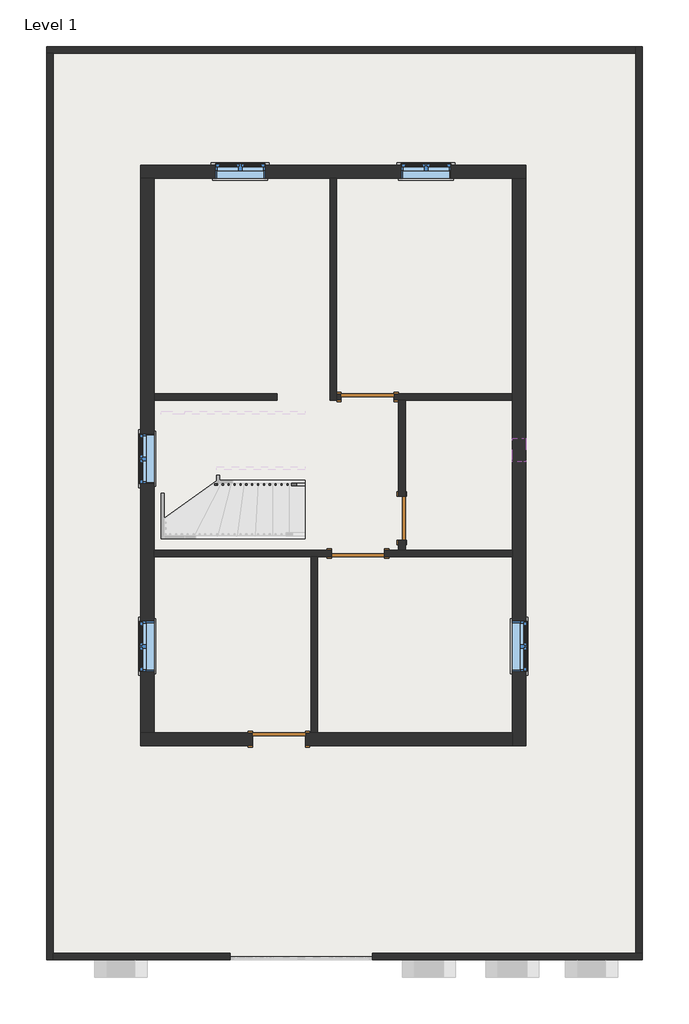
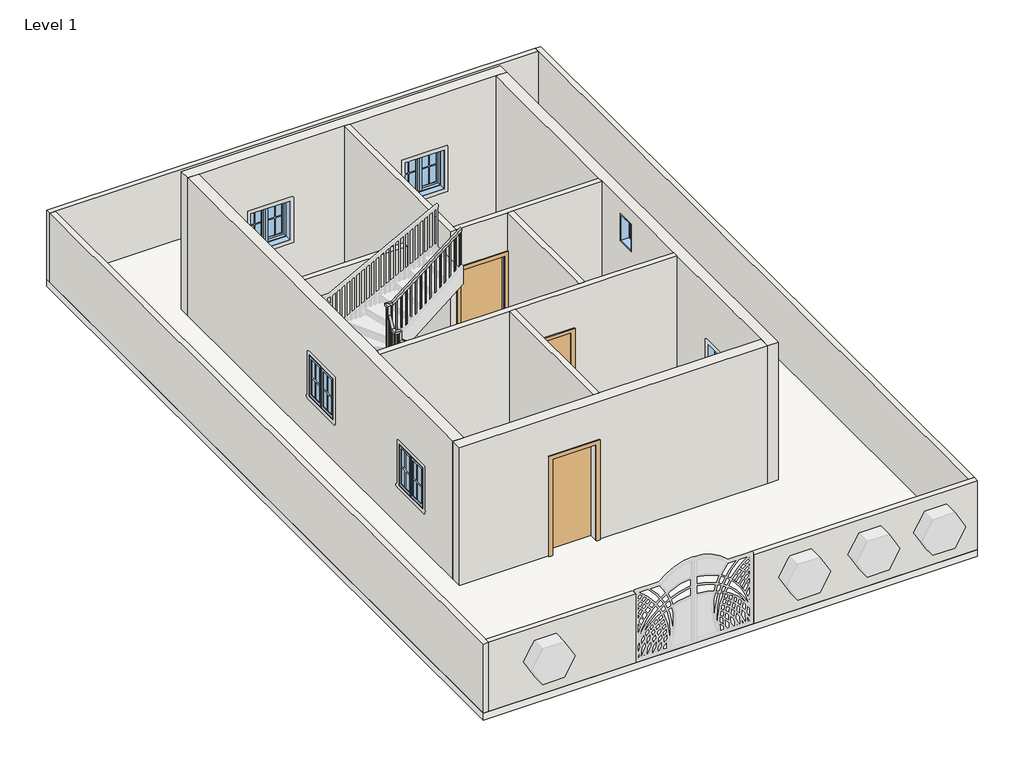
# One storey, part 1 of 2: 15 walls, 6 windows, 4 doors, 1 railing, 1 slab.
"""IFC4 building model written with IfcOpenShell, lengths in millimetres."""

from ifc_helpers import new_model, si_unit, frame, origin, origin_with_axes, place, context, project, spatial, polyline, outline, extrude, faceted_brep, transform, mapped, element, save
from components import door_d8f5dbb5, door_305aa2a5, door_e5f9f3c4, door_a90ba1ad, window_aa618e30, window_339605e1

model = new_model("IFC4")

# Units and contexts
model_context = context("Model", 3, world=origin())
ifc_project = project(units=[si_unit("LENGTHUNIT", "METRE", prefix="MILLI")], contexts=[model_context])

# Site, building, storey
site = spatial("IfcSite", under=ifc_project)
building = spatial("IfcBuilding", under=site)
storey = spatial("IfcBuildingStorey", under=building, Name="Level 1", Elevation=0.0)

# Doors
placement = place(None, origin())
door_shape = door_d8f5dbb5(model_context)
element("IfcDoor", 1, ObjectType="Single-Flush : 30\" x 80\"", at=placement, inside=storey, context=model_context, shape_type="MappedRepresentation", body=[
    mapped(door_shape, transform((-82.2715692, -955.3070853, 0.0), x_axis=(0.0, -1.0, 0.0), y_axis=(1.0, 0.0, 0.0), z_axis=(0.0, 0.0, 1.0))),
])
door_2_shape = door_305aa2a5(model_context)
element("IfcDoor", 2, ObjectType="Single-Flush : 36\" x 84\"", at=placement, inside=storey, context=model_context, shape_type="MappedRepresentation", body=[
    mapped(door_2_shape, transform((-677.5332429, 1140.1929147, 0.0), x_axis=(-1.0, 0.0, 0.0), y_axis=(0.0, -1.0, 0.0), z_axis=(0.0, 0.0, 1.0))),
])
door_3_shape = door_e5f9f3c4(model_context)
element("IfcDoor", 3, ObjectType="Single-Flush : 36\" x 84\"", at=placement, inside=storey, context=model_context, shape_type="MappedRepresentation", body=[
    mapped(door_3_shape, transform((-842.6332429, -1564.9070853, 0.0), x_axis=(-1.0, 0.0, 0.0), y_axis=(0.0, -1.0, 0.0), z_axis=(0.0, 0.0, 1.0))),
])
door_4_shape = door_a90ba1ad(model_context)
element("IfcDoor", 4, ObjectType="Single-Flush : 36\" x 84\"", at=placement, inside=storey, context=model_context, shape_type="MappedRepresentation", body=[
    mapped(door_4_shape, transform((-2212.5949167, -4784.3570853, 0.0), x_axis=(-1.0, 0.0, 0.0), y_axis=(0.0, -1.0, 0.0), z_axis=(0.0, 0.0, 1.0))),
])

# Railing
element("IfcRailing", 5, ObjectType="Handrail - Rectangular", at=placement, inside=storey, context=model_context, shape_type="SolidModel", body=[
    faceted_brep([(-1761.7449167, -396.5070853, 1083.7333333), (-1761.7449167, -396.5070853, 1019.4000346), (-1761.7449167, -345.7070853, 1019.4000346), (-1761.7449167, -345.7070853, 1083.7333333), (-3213.2766085, -396.5070853, 2211.6191036), (-3264.0766085, -396.5070853, 2186.7590024), (-3264.0766085, -345.7070853, 2186.7590024), (-3213.2766085, -345.7070853, 2211.6191036), (-3213.2766085, -396.5070853, 2414.6281882), (-3264.0766085, -396.5070853, 2363.8281882), (-3264.0766085, -345.7070853, 2363.8281882), (-3213.2766085, -345.7070853, 2414.6281882), (-3340.2766085, -396.5070853, 2414.6281882), (-3340.2766085, -396.5070853, 2363.8281882), (-3289.4766085, -345.7070853, 2363.8281882), (-3289.4766085, -345.7070853, 2414.6281882), (-3340.2766085, -269.5070853, 2414.6281882), (-3340.2766085, -240.3857515, 2363.8281882), (-3289.4766085, -240.3857515, 2363.8281882), (-3289.4766085, -269.5070853, 2414.6281882), (-3340.2766085, -142.5070853, 2631.5051451), (-3340.2766085, -91.7070853, 2617.7256424), (-3289.4766085, -91.7070853, 2617.7256424), (-3289.4766085, -142.5070853, 2631.5051451), (-3340.2766085, -142.5070853, 2834.5142297), (-3340.2766085, -91.7070853, 2783.7142297), (-3289.4766085, -91.7070853, 2783.7142297), (-3289.4766085, -142.5070853, 2834.5142297), (-3340.2766085, -15.5070853, 2834.5142297), (-3340.2766085, -15.5070853, 2783.7142297), (-3289.4766085, -66.3070853, 2783.7142297), (-3289.4766085, -66.3070853, 2834.5142297), (-3213.2766085, -15.5070853, 2834.5142297), (-3195.8599406, -15.5070853, 2783.7142297), (-3195.8599406, -66.3070853, 2783.7142297), (-3213.2766085, -66.3070853, 2834.5142297), (-1761.7449167, -15.5070853, 3962.4), (-1761.7449167, -66.3070853, 3962.4), (-1761.7449167, -66.3070853, 3898.0667013), (-1761.7449167, -15.5070853, 3898.0667013)], [[[0, 1, 2, 3]], [[1, 0, 4, 5]], [[2, 1, 5, 6]], [[3, 2, 6, 7]], [[0, 3, 7, 4]], [[5, 4, 8, 9]], [[6, 5, 9, 10]], [[7, 6, 10, 11]], [[4, 7, 11, 8]], [[9, 8, 12, 13]], [[10, 9, 13, 14]], [[11, 10, 14, 15]], [[8, 11, 15, 12]], [[13, 12, 16, 17]], [[14, 13, 17, 18]], [[15, 14, 18, 19]], [[12, 15, 19, 16]], [[17, 16, 20, 21]], [[18, 17, 21, 22]], [[19, 18, 22, 23]], [[16, 19, 23, 20]], [[21, 20, 24, 25]], [[22, 21, 25, 26]], [[23, 22, 26, 27]], [[20, 23, 27, 24]], [[25, 24, 28, 29]], [[26, 25, 29, 30]], [[27, 26, 30, 31]], [[24, 27, 31, 28]], [[29, 28, 32, 33]], [[30, 29, 33, 34]], [[31, 30, 34, 35]], [[28, 31, 35, 32]], [[36, 37, 38, 39]], [[33, 32, 36, 39]], [[34, 33, 39, 38]], [[35, 34, 38, 37]], [[32, 35, 37, 36]]]),
    extrude(outline(polyline([(3882.8316852, -1781.3516085), (3868.0292361, -1800.4016085), (2878.6666667, -1800.4016085), (2878.6666667, -1781.3516085), (3882.8316852, -1781.3516085)])), frame((0.0, -50.4320853, 0.0), z_axis=(0.0, 1.0, 0.0), x_axis=(0.0, 0.0, 1.0)), (0.0, 0.0, 1.0), 19.05),
    extrude(outline(polyline([(3803.8852902, -1882.9516085), (3789.0828411, -1902.0016085), (2878.6666667, -1902.0016085), (2878.6666667, -1882.9516085), (3803.8852902, -1882.9516085)])), frame((0.0, -50.4320853, 0.0), z_axis=(0.0, 1.0, 0.0), x_axis=(0.0, 0.0, 1.0)), (0.0, 0.0, 1.0), 19.05),
    extrude(outline(polyline([(3724.9388952, -1984.5516085), (3710.1364462, -2003.6016085), (2878.6666667, -2003.6016085), (2878.6666667, -1984.5516085), (3724.9388952, -1984.5516085)])), frame((0.0, -50.4320853, 0.0), z_axis=(0.0, 1.0, 0.0), x_axis=(0.0, 0.0, 1.0)), (0.0, 0.0, 1.0), 19.05),
    extrude(outline(polyline([(3645.9925003, -2086.1516085), (3631.1900512, -2105.2016085), (2709.3333333, -2105.2016085), (2709.3333333, -2086.1516085), (3645.9925003, -2086.1516085)])), frame((0.0, -50.4320853, 0.0), z_axis=(0.0, 1.0, 0.0), x_axis=(0.0, 0.0, 1.0)), (0.0, 0.0, 1.0), 19.05),
    extrude(outline(polyline([(3567.0461053, -2187.7516085), (3552.2436562, -2206.8016085), (2709.3333333, -2206.8016085), (2709.3333333, -2187.7516085), (3567.0461053, -2187.7516085)])), frame((0.0, -50.4320853, 0.0), z_axis=(0.0, 1.0, 0.0), x_axis=(0.0, 0.0, 1.0)), (0.0, 0.0, 1.0), 19.05),
    extrude(outline(polyline([(3488.0997103, -2289.3516085), (3473.2972613, -2308.4016085), (2709.3333333, -2308.4016085), (2709.3333333, -2289.3516085), (3488.0997103, -2289.3516085)])), frame((0.0, -50.4320853, 0.0), z_axis=(0.0, 1.0, 0.0), x_axis=(0.0, 0.0, 1.0)), (0.0, 0.0, 1.0), 19.05),
    extrude(outline(polyline([(3409.1533154, -2390.9516085), (3394.3508663, -2410.0016085), (2540.0, -2410.0016085), (2540.0, -2390.9516085), (3409.1533154, -2390.9516085)])), frame((0.0, -50.4320853, 0.0), z_axis=(0.0, 1.0, 0.0), x_axis=(0.0, 0.0, 1.0)), (0.0, 0.0, 1.0), 19.05),
    extrude(outline(polyline([(3330.2069204, -2492.5516085), (3315.4044713, -2511.6016085), (2540.0, -2511.6016085), (2540.0, -2492.5516085), (3330.2069204, -2492.5516085)])), frame((0.0, -50.4320853, 0.0), z_axis=(0.0, 1.0, 0.0), x_axis=(0.0, 0.0, 1.0)), (0.0, 0.0, 1.0), 19.05),
    extrude(outline(polyline([(3251.2605254, -2594.1516085), (3236.4580764, -2613.2016085), (2370.6666667, -2613.2016085), (2370.6666667, -2594.1516085), (3251.2605254, -2594.1516085)])), frame((0.0, -50.4320853, 0.0), z_axis=(0.0, 1.0, 0.0), x_axis=(0.0, 0.0, 1.0)), (0.0, 0.0, 1.0), 19.05),
    extrude(outline(polyline([(3172.3141304, -2695.7516085), (3157.5116814, -2714.8016085), (2370.6666667, -2714.8016085), (2370.6666667, -2695.7516085), (3172.3141304, -2695.7516085)])), frame((0.0, -50.4320853, 0.0), z_axis=(0.0, 1.0, 0.0), x_axis=(0.0, 0.0, 1.0)), (0.0, 0.0, 1.0), 19.05),
    extrude(outline(polyline([(3093.3677355, -2797.3516085), (3078.5652864, -2816.4016085), (2370.6666667, -2816.4016085), (2370.6666667, -2797.3516085), (3093.3677355, -2797.3516085)])), frame((0.0, -50.4320853, 0.0), z_axis=(0.0, 1.0, 0.0), x_axis=(0.0, 0.0, 1.0)), (0.0, 0.0, 1.0), 19.05),
    extrude(outline(polyline([(3014.4213405, -2898.9516085), (2999.6188914, -2918.0016085), (2201.3333333, -2918.0016085), (2201.3333333, -2898.9516085), (3014.4213405, -2898.9516085)])), frame((0.0, -50.4320853, 0.0), z_axis=(0.0, 1.0, 0.0), x_axis=(0.0, 0.0, 1.0)), (0.0, 0.0, 1.0), 19.05),
    extrude(outline(polyline([(2935.4749455, -3000.5516085), (2920.6724965, -3019.6016085), (2201.3333333, -3019.6016085), (2201.3333333, -3000.5516085), (2935.4749455, -3000.5516085)])), frame((0.0, -50.4320853, 0.0), z_axis=(0.0, 1.0, 0.0), x_axis=(0.0, 0.0, 1.0)), (0.0, 0.0, 1.0), 19.05),
    extrude(outline(polyline([(2856.5285506, -3102.1516085), (2841.7261015, -3121.2016085), (2032.0, -3121.2016085), (2032.0, -3102.1516085), (2856.5285506, -3102.1516085)])), frame((0.0, -50.4320853, 0.0), z_axis=(0.0, 1.0, 0.0), x_axis=(0.0, 0.0, 1.0)), (0.0, 0.0, 1.0), 19.05),
    extrude(outline(polyline([(2777.5821556, -3203.7516085), (2762.7797065, -3222.8016085), (2032.0, -3222.8016085), (2032.0, -3203.7516085), (2777.5821556, -3203.7516085)])), frame((0.0, -50.4320853, 0.0), z_axis=(0.0, 1.0, 0.0), x_axis=(0.0, 0.0, 1.0)), (0.0, 0.0, 1.0), 19.05),
    extrude(outline(polyline([(-3305.3516085, -75.8320853), (-3324.4016085, -75.8320853), (-3324.4016085, -56.7820853), (-3305.3516085, -56.7820853), (-3305.3516085, -75.8320853)])), frame((0.0, 0.0, 1693.3333333), z_axis=(0.0, 0.0, 1.0), x_axis=(1.0, 0.0, 0.0)), (0.0, 0.0, 1.0), 1090.3808964),
    extrude(outline(polyline([(-177.4320853, 2471.3336964), (-158.3820853, 2503.86524), (-158.3820853, 1524.0), (-177.4320853, 1524.0), (-177.4320853, 2471.3336964)])), frame((-3324.4016085, 0.0, 0.0), z_axis=(1.0, 0.0, 0.0), x_axis=(0.0, 1.0, 0.0)), (0.0, 0.0, 1.0), 19.05),
    extrude(outline(polyline([(-279.0320853, 2297.8321309), (-259.9820853, 2330.3636744), (-259.9820853, 1354.6666667), (-279.0320853, 1354.6666667), (-279.0320853, 2297.8321309)])), frame((-3324.4016085, 0.0, 0.0), z_axis=(1.0, 0.0, 0.0), x_axis=(0.0, 1.0, 0.0)), (0.0, 0.0, 1.0), 19.05),
    extrude(outline(polyline([(-3276.2199167, -361.5820853), (-3276.2199167, -380.6320853), (-3295.2699167, -380.6320853), (-3295.2699167, -361.5820853), (-3276.2199167, -361.5820853)])), frame((0.0, 0.0, 1185.3333333), z_axis=(0.0, 0.0, 1.0), x_axis=(1.0, 0.0, 0.0)), (0.0, 0.0, 1.0), 1178.4948549),
    extrude(outline(polyline([(2117.2483397, -3174.6199167), (2132.0507888, -3193.6699167), (1016.0, -3193.6699167), (1016.0, -3174.6199167), (2117.2483397, -3174.6199167)])), frame((0.0, -380.6320853, 0.0), z_axis=(0.0, 1.0, 0.0), x_axis=(0.0, 0.0, 1.0)), (0.0, 0.0, 1.0), 19.05),
    extrude(outline(polyline([(2038.3019447, -3073.0199167), (2053.1043938, -3092.0699167), (1016.0, -3092.0699167), (1016.0, -3073.0199167), (2038.3019447, -3073.0199167)])), frame((0.0, -380.6320853, 0.0), z_axis=(0.0, 1.0, 0.0), x_axis=(0.0, 0.0, 1.0)), (0.0, 0.0, 1.0), 19.05),
    extrude(outline(polyline([(1959.3555498, -2971.4199167), (1974.1579988, -2990.4699167), (846.6666667, -2990.4699167), (846.6666667, -2971.4199167), (1959.3555498, -2971.4199167)])), frame((0.0, -380.6320853, 0.0), z_axis=(0.0, 1.0, 0.0), x_axis=(0.0, 0.0, 1.0)), (0.0, 0.0, 1.0), 19.05),
    extrude(outline(polyline([(1880.4091548, -2869.8199167), (1895.2116039, -2888.8699167), (846.6666667, -2888.8699167), (846.6666667, -2869.8199167), (1880.4091548, -2869.8199167)])), frame((0.0, -380.6320853, 0.0), z_axis=(0.0, 1.0, 0.0), x_axis=(0.0, 0.0, 1.0)), (0.0, 0.0, 1.0), 19.05),
    extrude(outline(polyline([(1801.4627598, -2768.2199167), (1816.2652089, -2787.2699167), (677.3333333, -2787.2699167), (677.3333333, -2768.2199167), (1801.4627598, -2768.2199167)])), frame((0.0, -380.6320853, 0.0), z_axis=(0.0, 1.0, 0.0), x_axis=(0.0, 0.0, 1.0)), (0.0, 0.0, 1.0), 19.05),
    extrude(outline(polyline([(1722.5163649, -2666.6199167), (1737.3188139, -2685.6699167), (677.3333333, -2685.6699167), (677.3333333, -2666.6199167), (1722.5163649, -2666.6199167)])), frame((0.0, -380.6320853, 0.0), z_axis=(0.0, 1.0, 0.0), x_axis=(0.0, 0.0, 1.0)), (0.0, 0.0, 1.0), 19.05),
    extrude(outline(polyline([(1643.5699699, -2565.0199167), (1658.3724189, -2584.0699167), (508.0, -2584.0699167), (508.0, -2565.0199167), (1643.5699699, -2565.0199167)])), frame((0.0, -380.6320853, 0.0), z_axis=(0.0, 1.0, 0.0), x_axis=(0.0, 0.0, 1.0)), (0.0, 0.0, 1.0), 19.05),
    extrude(outline(polyline([(1564.6235749, -2463.4199167), (1579.426024, -2482.4699167), (508.0, -2482.4699167), (508.0, -2463.4199167), (1564.6235749, -2463.4199167)])), frame((0.0, -380.6320853, 0.0), z_axis=(0.0, 1.0, 0.0), x_axis=(0.0, 0.0, 1.0)), (0.0, 0.0, 1.0), 19.05),
    extrude(outline(polyline([(1485.6771799, -2361.8199167), (1500.479629, -2380.8699167), (508.0, -2380.8699167), (508.0, -2361.8199167), (1485.6771799, -2361.8199167)])), frame((0.0, -380.6320853, 0.0), z_axis=(0.0, 1.0, 0.0), x_axis=(0.0, 0.0, 1.0)), (0.0, 0.0, 1.0), 19.05),
    extrude(outline(polyline([(1406.730785, -2260.2199167), (1421.533234, -2279.2699167), (338.6666667, -2279.2699167), (338.6666667, -2260.2199167), (1406.730785, -2260.2199167)])), frame((0.0, -380.6320853, 0.0), z_axis=(0.0, 1.0, 0.0), x_axis=(0.0, 0.0, 1.0)), (0.0, 0.0, 1.0), 19.05),
    extrude(outline(polyline([(1327.78439, -2158.6199167), (1342.5868391, -2177.6699167), (338.6666667, -2177.6699167), (338.6666667, -2158.6199167), (1327.78439, -2158.6199167)])), frame((0.0, -380.6320853, 0.0), z_axis=(0.0, 1.0, 0.0), x_axis=(0.0, 0.0, 1.0)), (0.0, 0.0, 1.0), 19.05),
    extrude(outline(polyline([(1248.837995, -2057.0199167), (1263.6404441, -2076.0699167), (338.6666667, -2076.0699167), (338.6666667, -2057.0199167), (1248.837995, -2057.0199167)])), frame((0.0, -380.6320853, 0.0), z_axis=(0.0, 1.0, 0.0), x_axis=(0.0, 0.0, 1.0)), (0.0, 0.0, 1.0), 19.05),
    extrude(outline(polyline([(1169.8916001, -1955.4199167), (1184.6940491, -1974.4699167), (169.3333333, -1974.4699167), (169.3333333, -1955.4199167), (1169.8916001, -1955.4199167)])), frame((0.0, -380.6320853, 0.0), z_axis=(0.0, 1.0, 0.0), x_axis=(0.0, 0.0, 1.0)), (0.0, 0.0, 1.0), 19.05),
    extrude(outline(polyline([(1090.9452051, -1853.8199167), (1105.7476541, -1872.8699167), (169.3333333, -1872.8699167), (169.3333333, -1853.8199167), (1090.9452051, -1853.8199167)])), frame((0.0, -380.6320853, 0.0), z_axis=(0.0, 1.0, 0.0), x_axis=(0.0, 0.0, 1.0)), (0.0, 0.0, 1.0), 19.05),
    extrude(outline(polyline([(-3305.3516085, -50.4320853), (-3324.4016085, -50.4320853), (-3324.4016085, -31.3820853), (-3305.3516085, -31.3820853), (-3305.3516085, -50.4320853)])), frame((0.0, 0.0, 1862.6666667), z_axis=(0.0, 0.0, 1.0), x_axis=(1.0, 0.0, 0.0)), (0.0, 0.0, 1.0), 921.0475631),
    extrude(outline(polyline([(-3305.3516085, -361.5820853), (-3305.3516085, -380.6320853), (-3324.4016085, -380.6320853), (-3324.4016085, -361.5820853), (-3305.3516085, -361.5820853)])), frame((0.0, 0.0, 1185.3333333), z_axis=(0.0, 0.0, 1.0), x_axis=(1.0, 0.0, 0.0)), (0.0, 0.0, 1.0), 1178.4948549),
    extrude(outline(polyline([(3898.0667013, -1761.7449167), (3883.2642523, -1780.7949167), (2878.6666667, -1780.7949167), (2878.6666667, -1761.7449167), (3898.0667013, -1761.7449167)])), frame((0.0, -50.4320853, 0.0), z_axis=(0.0, 1.0, 0.0), x_axis=(0.0, 0.0, 1.0)), (0.0, 0.0, 1.0), 19.05),
    extrude(outline(polyline([(1019.4000346, -1761.7449167), (1034.2024837, -1780.7949167), (169.3333333, -1780.7949167), (169.3333333, -1761.7449167), (1019.4000346, -1761.7449167)])), frame((0.0, -380.6320853, 0.0), z_axis=(0.0, 1.0, 0.0), x_axis=(0.0, 0.0, 1.0)), (0.0, 0.0, 1.0), 19.05),
])

# Slab
element("IfcSlab", 6, ObjectType="Generic - 12\"", at=placement, inside=storey, context=model_context, shape_type="SweptSolid", body=[
    extrude(outline(polyline([(4085.235039, 7210.558909), (4085.235039, -8600.941091), (-6239.864961, -8600.941091), (-6239.864961, 7210.558909), (4085.235039, 7210.558909)])), frame((0.0, 0.0, -152.4), z_axis=(0.0, 0.0, 1.0), x_axis=(1.0, 0.0, 0.0)), (0.0, 0.0, 1.0), 152.4),
])

# Walls
element("IfcWall", 7, ObjectType="WALL4.5\"", at=placement, inside=storey, context=model_context, shape_type="Brep", body=[
    faceted_brep([(-1329.9449167, 4931.1429147, 0.0), (-1329.9449167, 1083.0429147, 0.0), (-1329.9449167, 1083.0429147, 3048.0), (-1329.9449167, 4931.1429147, 3048.0), (-1215.6449167, 4931.1429147, 0.0), (-1215.6449167, 4931.1429147, 3048.0), (-1215.6449167, 1197.3429147, 3048.0), (-1215.6449167, 1083.0429147, 3048.0), (-1215.6449167, 1083.0429147, 0.0), (-1215.6449167, 1197.3429147, 0.0)], [[[0, 1, 2, 3]], [[4, 5, 6, 7, 8, 9]], [[1, 0, 4, 9, 8]], [[0, 3, 5, 4]], [[2, 1, 8, 7]], [[3, 2, 7, 6, 5]]]),
])
element("IfcWall", 8, ObjectType="WALL4.5\"", at=placement, inside=storey, context=model_context, shape_type="Brep", body=[
    faceted_brep([(-1215.6449167, 1083.0429147, 0.0), (-1134.7332429, 1083.0429147, 0.0), (-1134.7332429, 1083.0429147, 2133.6), (-220.3332429, 1083.0429147, 2133.6), (-220.3332429, 1083.0429147, 0.0), (-139.4215692, 1083.0429147, 0.0), (-25.1215692, 1083.0429147, 0.0), (1832.3550833, 1083.0429147, 0.0), (1832.3550833, 1083.0429147, 3048.0), (-25.1215692, 1083.0429147, 3048.0), (-139.4215692, 1083.0429147, 3048.0), (-1215.6449167, 1083.0429147, 3048.0), (-1134.7332429, 1197.3429147, 2133.6), (-1134.7332429, 1197.3429147, 0.0), (-1215.6449167, 1197.3429147, 0.0), (-1215.6449167, 1197.3429147, 3048.0), (1832.3550833, 1197.3429147, 3048.0), (1832.3550833, 1197.3429147, 0.0), (-220.3332429, 1197.3429147, 0.0), (-220.3332429, 1197.3429147, 2133.6)], [[[0, 1, 2, 3, 4, 5, 6, 7, 8, 9, 10, 11]], [[12, 13, 14, 15, 16, 17, 18, 19]], [[18, 17, 7, 6, 5, 4]], [[14, 13, 1, 0]], [[0, 11, 15, 14]], [[8, 7, 17, 16]], [[2, 1, 13, 12]], [[3, 2, 12, 19]], [[4, 3, 19, 18]], [[11, 10, 9, 8, 16, 15]]]),
])
element("IfcWall", 9, ObjectType="WALL4.5\"", at=placement, inside=storey, context=model_context, shape_type="SweptSolid", body=[
    extrude(outline(polyline([(-2244.3449167, 1083.0429147), (-4377.9449167, 1083.0429147), (-4377.9449167, 1197.3429147), (-2244.3449167, 1197.3429147), (-2244.3449167, 1083.0429147)])), origin_with_axes(), (0.0, 0.0, 1.0), 3048.0),
])
element("IfcWall", 10, ObjectType="WALL4.5\"", at=placement, inside=storey, context=model_context, shape_type="SweptSolid", body=[
    extrude(outline(polyline([(-1336.3070853, 2032.0), (-1336.3070853, 0.0), (-1507.7570853, 0.0), (-1507.7570853, 3048.0), (1083.0429147, 3048.0), (1083.0429147, 0.0), (-574.3070853, 0.0), (-574.3070853, 2032.0), (-1336.3070853, 2032.0)])), frame((-139.4215692, 0.0, 0.0), z_axis=(1.0, 0.0, 0.0), x_axis=(0.0, 1.0, 0.0)), (0.0, 0.0, 1.0), 114.3),
])
element("IfcWall", 11, ObjectType="WALL4.5\"", at=placement, inside=storey, context=model_context, shape_type="Brep", body=[
    faceted_brep([(-4377.9449167, -1622.0570853, 0.0), (-1660.1449167, -1622.0570853, 0.0), (-1545.8449167, -1622.0570853, 0.0), (-1299.8332429, -1622.0570853, 0.0), (-1299.8332429, -1622.0570853, 2133.6), (-385.4332429, -1622.0570853, 2133.6), (-385.4332429, -1622.0570853, 0.0), (1832.3550833, -1622.0570853, 0.0), (1832.3550833, -1622.0570853, 3048.0), (-1545.8449167, -1622.0570853, 3048.0), (-1660.1449167, -1622.0570853, 3048.0), (-4377.9449167, -1622.0570853, 3048.0), (-1299.8332429, -1507.7570853, 2133.6), (-1299.8332429, -1507.7570853, 0.0), (-4377.9449167, -1507.7570853, 0.0), (-4377.9449167, -1507.7570853, 3048.0), (-139.4215692, -1507.7570853, 3048.0), (-25.1215692, -1507.7570853, 3048.0), (1832.3550833, -1507.7570853, 3048.0), (1832.3550833, -1507.7570853, 0.0), (-25.1215692, -1507.7570853, 0.0), (-139.4215692, -1507.7570853, 0.0), (-385.4332429, -1507.7570853, 0.0), (-385.4332429, -1507.7570853, 2133.6)], [[[0, 1, 2, 3, 4, 5, 6, 7, 8, 9, 10, 11]], [[12, 13, 14, 15, 16, 17, 18, 19, 20, 21, 22, 23]], [[14, 13, 3, 2, 1, 0]], [[22, 21, 20, 19, 7, 6]], [[8, 7, 19, 18]], [[0, 11, 15, 14]], [[4, 3, 13, 12]], [[5, 4, 12, 23]], [[6, 5, 23, 22]], [[11, 10, 9, 8, 18, 17, 16, 15]]]),
])
element("IfcWall", 12, ObjectType="WALL4.5\"", at=placement, inside=storey, context=model_context, shape_type="SweptSolid", body=[
    extrude(outline(polyline([(-1660.1449167, -4670.0570853), (-1660.1449167, -1622.0570853), (-1545.8449167, -1622.0570853), (-1545.8449167, -4670.0570853), (-1660.1449167, -4670.0570853)])), origin_with_axes(), (0.0, 0.0, 1.0), 3048.0),
])
element("IfcWall", 13, ObjectType="WALL4.5\"", at=placement, inside=storey, context=model_context, shape_type="Brep", body=[
    faceted_brep([(-6239.864961, 7096.258909, 0.0), (-6125.564961, 7096.258909, 0.0), (3970.935039, 7096.258909, 0.0), (3970.935039, 7096.258909, 1524.0), (-6125.564961, 7096.258909, 1524.0), (-6239.864961, 7096.258909, 1524.0), (-6239.864961, 7210.558909, 0.0), (-6239.864961, 7210.558909, 1524.0), (3970.935039, 7210.558909, 1524.0), (3970.935039, 7210.558909, 0.0)], [[[0, 1, 2, 3, 4, 5]], [[6, 7, 8, 9]], [[2, 1, 0, 6, 9]], [[5, 4, 3, 8, 7]], [[0, 5, 7, 6]], [[3, 2, 9, 8]]]),
])
element("IfcWall", 14, ObjectType="WALL4.5\"", at=placement, inside=storey, context=model_context, shape_type="Brep", body=[
    faceted_brep([(-6125.564961, -8600.941091, 0.0), (-6125.564961, -8486.641091, 0.0), (-6125.564961, 7096.258909, 0.0), (-6125.564961, 7096.258909, 1524.0), (-6125.564961, -8486.641091, 1524.0), (-6125.564961, -8600.941091, 1524.0), (-6239.864961, -8600.941091, 0.0), (-6239.864961, -8600.941091, 1524.0), (-6239.864961, 7096.258909, 1524.0), (-6239.864961, 7096.258909, 0.0)], [[[0, 1, 2, 3, 4, 5]], [[6, 7, 8, 9]], [[2, 1, 0, 6, 9]], [[5, 4, 3, 8, 7]], [[0, 5, 7, 6]], [[3, 2, 9, 8]]]),
])
element("IfcWall", 15, ObjectType="WALL4.5\"", at=placement, inside=storey, context=model_context, shape_type="Brep", body=[
    faceted_brep([(4085.235039, -8486.641091, 0.0), (3970.935039, -8486.641091, 0.0), (-594.714961, -8486.641091, 0.0), (-594.714961, -8486.641091, 1524.0), (3970.935039, -8486.641091, 1524.0), (4085.235039, -8486.641091, 1524.0), (4085.235039, -8600.941091, 0.0), (4085.235039, -8600.941091, 1524.0), (-594.714961, -8600.941091, 1524.0), (-594.714961, -8600.941091, 0.0)], [[[0, 1, 2, 3, 4, 5]], [[6, 7, 8, 9]], [[2, 1, 0, 6, 9]], [[3, 2, 9, 8]], [[5, 4, 3, 8, 7]], [[0, 5, 7, 6]]]),
])
element("IfcWall", 16, ObjectType="WALL4.5\"", at=placement, inside=storey, context=model_context, shape_type="Brep", body=[
    faceted_brep([(3970.935039, 7210.558909, 0.0), (3970.935039, 7096.258909, 0.0), (3970.935039, -8486.641091, 0.0), (3970.935039, -8486.641091, 1524.0), (3970.935039, 7096.258909, 1524.0), (3970.935039, 7210.558909, 1524.0), (4085.235039, 7210.558909, 0.0), (4085.235039, 7210.558909, 1524.0), (4085.235039, -8486.641091, 1524.0), (4085.235039, -8486.641091, 0.0)], [[[0, 1, 2, 3, 4, 5]], [[6, 7, 8, 9]], [[2, 1, 0, 6, 9]], [[5, 4, 3, 8, 7]], [[0, 5, 7, 6]], [[3, 2, 9, 8]]]),
])
element("IfcWall", 17, ObjectType="WALL4.5\"", at=placement, inside=storey, context=model_context, shape_type="SweptSolid", body=[
    extrude(outline(polyline([(-6125.564961, -8486.641091), (-3058.514961, -8486.641091), (-3058.514961, -8600.941091), (-6125.564961, -8600.941091), (-6125.564961, -8486.641091)])), origin_with_axes(), (0.0, 0.0, 1.0), 1524.0),
])
element("IfcWall", 18, ObjectType="WALL9\"", at=placement, inside=storey, context=model_context, shape_type="Brep", body=[
    faceted_brep([(-4606.5449167, 4931.1429147, 0.0), (-4377.9449167, 4931.1429147, 0.0), (-1329.9449167, 4931.1429147, 0.0), (-1215.6449167, 4931.1429147, 0.0), (1832.3550833, 4931.1429147, 0.0), (2060.9550833, 4931.1429147, 0.0), (2060.9550833, 4931.1429147, 3048.0), (1832.3550833, 4931.1429147, 3048.0), (-1215.6449167, 4931.1429147, 3048.0), (-1329.9449167, 4931.1429147, 3048.0), (-4377.9449167, 4931.1429147, 3048.0), (-4606.5449167, 4931.1429147, 3048.0), (-2450.7199167, 4931.1429147, 1828.8), (-2450.7199167, 4931.1429147, 914.4), (-3314.3199167, 4931.1429147, 914.4), (-3314.3199167, 4931.1429147, 1828.8), (768.7300833, 4931.1429147, 1828.8), (768.7300833, 4931.1429147, 914.4), (-94.8699167, 4931.1429147, 914.4), (-94.8699167, 4931.1429147, 1828.8), (-4606.5449167, 5159.7429147, 0.0), (-4606.5449167, 5159.7429147, 3048.0), (2060.9550833, 5159.7429147, 3048.0), (2060.9550833, 5159.7429147, 0.0), (-2450.7199167, 5159.7429147, 1828.8), (-3314.3199167, 5159.7429147, 1828.8), (-3314.3199167, 5159.7429147, 914.4), (-2450.7199167, 5159.7429147, 914.4), (768.7300833, 5159.7429147, 1828.8), (-94.8699167, 5159.7429147, 1828.8), (-94.8699167, 5159.7429147, 914.4), (768.7300833, 5159.7429147, 914.4)], [[[0, 1, 2, 3, 4, 5, 6, 7, 8, 9, 10, 11], [12, 13, 14, 15], [16, 17, 18, 19]], [[20, 21, 22, 23], [24, 25, 26, 27], [28, 29, 30, 31]], [[5, 4, 3, 2, 1, 0, 20, 23]], [[6, 5, 23, 22]], [[0, 11, 21, 20]], [[13, 12, 24, 27]], [[14, 13, 27, 26]], [[15, 14, 26, 25]], [[12, 15, 25, 24]], [[17, 16, 28, 31]], [[18, 17, 31, 30]], [[19, 18, 30, 29]], [[16, 19, 29, 28]], [[11, 10, 9, 8, 7, 6, 22, 21]]]),
])
element("IfcWall", 19, ObjectType="WALL9\"", at=placement, inside=storey, context=model_context, shape_type="Brep", body=[
    faceted_brep([(1832.3550833, 4931.1429147, 0.0), (1832.3550833, 1197.3429147, 0.0), (1832.3550833, 1083.0429147, 0.0), (1832.3550833, -1507.7570853, 0.0), (1832.3550833, -1622.0570853, 0.0), (1832.3550833, -4670.0570853, 0.0), (1832.3550833, -4898.6570853, 0.0), (1832.3550833, -4898.6570853, 3048.0), (1832.3550833, -4670.0570853, 3048.0), (1832.3550833, -1622.0570853, 3048.0), (1832.3550833, -1507.7570853, 3048.0), (1832.3550833, 1083.0429147, 3048.0), (1832.3550833, 1197.3429147, 3048.0), (1832.3550833, 4931.1429147, 3048.0), (1832.3550833, 22.5929147, 2743.2), (1832.3550833, 22.5929147, 2133.6), (1832.3550833, 428.9929147, 2133.6), (1832.3550833, 428.9929147, 2743.2), (1832.3550833, -3606.4320853, 1828.8), (1832.3550833, -3606.4320853, 914.4), (1832.3550833, -2742.8320853, 914.4), (1832.3550833, -2742.8320853, 1828.8), (2060.9550833, 4931.1429147, 0.0), (2060.9550833, 4931.1429147, 3048.0), (2060.9550833, -4898.6570853, 3048.0), (2060.9550833, -4898.6570853, 0.0), (2060.9550833, 22.5929147, 2743.2), (2060.9550833, 428.9929147, 2743.2), (2060.9550833, 428.9929147, 2133.6), (2060.9550833, 22.5929147, 2133.6), (2060.9550833, -3606.4320853, 1828.8), (2060.9550833, -2742.8320853, 1828.8), (2060.9550833, -2742.8320853, 914.4), (2060.9550833, -3606.4320853, 914.4)], [[[0, 1, 2, 3, 4, 5, 6, 7, 8, 9, 10, 11, 12, 13], [14, 15, 16, 17], [18, 19, 20, 21]], [[22, 23, 24, 25], [26, 27, 28, 29], [30, 31, 32, 33]], [[6, 5, 4, 3, 2, 1, 0, 22, 25]], [[0, 13, 23, 22]], [[7, 6, 25, 24]], [[15, 14, 26, 29]], [[16, 15, 29, 28]], [[17, 16, 28, 27]], [[14, 17, 27, 26]], [[19, 18, 30, 33]], [[20, 19, 33, 32]], [[21, 20, 32, 31]], [[18, 21, 31, 30]], [[13, 12, 11, 10, 9, 8, 7, 24, 23]]]),
])
element("IfcWall", 20, ObjectType="WALL9\"", at=placement, inside=storey, context=model_context, shape_type="Brep", body=[
    faceted_brep([(-2669.7949167, -4670.0570853, 2133.6), (-2669.7949167, -4670.0570853, 0.0), (-4377.9449167, -4670.0570853, 0.0), (-4606.5449167, -4670.0570853, 0.0), (-4606.5449167, -4670.0570853, 3048.0), (-4377.9449167, -4670.0570853, 3048.0), (-1660.1449167, -4670.0570853, 3048.0), (-1545.8449167, -4670.0570853, 3048.0), (1832.3550833, -4670.0570853, 3048.0), (1832.3550833, -4670.0570853, 0.0), (-1545.8449167, -4670.0570853, 0.0), (-1660.1449167, -4670.0570853, 0.0), (-1755.3949167, -4670.0570853, 0.0), (-1755.3949167, -4670.0570853, 2133.6), (-4606.5449167, -4898.6570853, 0.0), (-2669.7949167, -4898.6570853, 0.0), (-2669.7949167, -4898.6570853, 2133.6), (-1755.3949167, -4898.6570853, 2133.6), (-1755.3949167, -4898.6570853, 0.0), (1832.3550833, -4898.6570853, 0.0), (1832.3550833, -4898.6570853, 3048.0), (-4606.5449167, -4898.6570853, 3048.0)], [[[0, 1, 2, 3, 4, 5, 6, 7, 8, 9, 10, 11, 12, 13]], [[14, 15, 16, 17, 18, 19, 20, 21]], [[3, 2, 1, 15, 14]], [[12, 11, 10, 9, 19, 18]], [[9, 8, 20, 19]], [[4, 3, 14, 21]], [[16, 15, 1, 0]], [[17, 16, 0, 13]], [[18, 17, 13, 12]], [[8, 7, 6, 5, 4, 21, 20]]]),
])
element("IfcWall", 21, ObjectType="WALL9\"", at=placement, inside=storey, context=model_context, shape_type="Brep", body=[
    faceted_brep([(-4377.9449167, -4670.0570853, 0.0), (-4377.9449167, -1622.0570853, 0.0), (-4377.9449167, -1507.7570853, 0.0), (-4377.9449167, 1083.0429147, 0.0), (-4377.9449167, 1197.3429147, 0.0), (-4377.9449167, 4931.1429147, 0.0), (-4377.9449167, 4931.1429147, 3048.0), (-4377.9449167, 1197.3429147, 3048.0), (-4377.9449167, 1083.0429147, 3048.0), (-4377.9449167, -1507.7570853, 3048.0), (-4377.9449167, -1622.0570853, 3048.0), (-4377.9449167, -4670.0570853, 3048.0), (-4377.9449167, -2742.8320853, 1828.8), (-4377.9449167, -2742.8320853, 914.4), (-4377.9449167, -3606.4320853, 914.4), (-4377.9449167, -3606.4320853, 1828.8), (-4377.9449167, 505.1929147, 1828.8), (-4377.9449167, 505.1929147, 914.4), (-4377.9449167, -358.4070853, 914.4), (-4377.9449167, -358.4070853, 1828.8), (-4606.5449167, -4670.0570853, 0.0), (-4606.5449167, -4670.0570853, 3048.0), (-4606.5449167, 4931.1429147, 3048.0), (-4606.5449167, 4931.1429147, 0.0), (-4606.5449167, -2742.8320853, 1828.8), (-4606.5449167, -3606.4320853, 1828.8), (-4606.5449167, -3606.4320853, 914.4), (-4606.5449167, -2742.8320853, 914.4), (-4606.5449167, 505.1929147, 1828.8), (-4606.5449167, -358.4070853, 1828.8), (-4606.5449167, -358.4070853, 914.4), (-4606.5449167, 505.1929147, 914.4)], [[[0, 1, 2, 3, 4, 5, 6, 7, 8, 9, 10, 11], [12, 13, 14, 15], [16, 17, 18, 19]], [[20, 21, 22, 23], [24, 25, 26, 27], [28, 29, 30, 31]], [[5, 4, 3, 2, 1, 0, 20, 23]], [[0, 11, 21, 20]], [[6, 5, 23, 22]], [[13, 12, 24, 27]], [[14, 13, 27, 26]], [[15, 14, 26, 25]], [[12, 15, 25, 24]], [[17, 16, 28, 31]], [[18, 17, 31, 30]], [[19, 18, 30, 29]], [[16, 19, 29, 28]], [[11, 10, 9, 8, 7, 6, 22, 21]]]),
])

# Windows
window_shape = window_aa618e30(model_context)
element("IfcWindow", 22, ObjectType="Fixed : 16\" x 24\"", at=placement, inside=storey, context=model_context, shape_type="MappedRepresentation", body=[
    mapped(window_shape, transform((1946.6550833, 187.6929147, 1219.2), x_axis=(0.0, -1.0, 0.0), y_axis=(1.0, 0.0, 0.0), z_axis=(0.0, 0.0, 1.0))),
])
window_2_shape = window_339605e1(model_context)
element("IfcWindow", 23, ObjectType="Window-Casement-Double : 34\" x 36\"", at=placement, inside=storey, context=model_context, shape_type="MappedRepresentation", body=[
    mapped(window_2_shape, transform((-2882.5199167, 5045.4429147, 0.0), x_axis=(1.0, 0.0, 0.0), y_axis=(0.0, 1.0, 0.0), z_axis=(0.0, 0.0, 1.0))),
])
element("IfcWindow", 24, ObjectType="Window-Casement-Double : 34\" x 36\"", at=placement, inside=storey, context=model_context, shape_type="MappedRepresentation", body=[
    mapped(window_2_shape, transform((336.9300833, 5045.4429147, 0.0), x_axis=(1.0, 0.0, 0.0), y_axis=(0.0, 1.0, 0.0), z_axis=(0.0, 0.0, 1.0))),
])
element("IfcWindow", 25, ObjectType="Window-Casement-Double : 34\" x 36\"", at=placement, inside=storey, context=model_context, shape_type="MappedRepresentation", body=[
    mapped(window_2_shape, transform((-4492.2449167, -3174.6320853, 0.0), x_axis=(0.0, 1.0, 0.0), y_axis=(-1.0, 0.0, 0.0), z_axis=(0.0, 0.0, 1.0))),
])
element("IfcWindow", 26, ObjectType="Window-Casement-Double : 34\" x 36\"", at=placement, inside=storey, context=model_context, shape_type="MappedRepresentation", body=[
    mapped(window_2_shape, transform((1946.6550833, -3174.6320853, 0.0), x_axis=(0.0, -1.0, 0.0), y_axis=(1.0, 0.0, 0.0), z_axis=(0.0, 0.0, 1.0))),
])
element("IfcWindow", 27, ObjectType="Window-Casement-Double : 34\" x 36\"", at=placement, inside=storey, context=model_context, shape_type="MappedRepresentation", body=[
    mapped(window_2_shape, transform((-4492.2449167, 73.3929147, 0.0), x_axis=(0.0, 1.0, 0.0), y_axis=(-1.0, 0.0, 0.0), z_axis=(0.0, 0.0, 1.0))),
])

save(model, "model.ifc")

# Revit data of these elements
# Type "Single-Flush : 30\" x 80\""
#   Type Mark = "5"
#   Construction Type Id = "MDOOR"
#   Assembly Code = "C1020"
#   Analytic Construction = "Metal"
#   Thickness = 0' - 2"
#   Heat Transfer Coefficient (U) = 0.651978 BTU/(h·ft²·°F)
#   Height = 6' - 8"
#   Trim Projection Ext = 0' - 1"
#   Trim Projection Int = 0' - 1"
#   Trim Width = 0' - 3"
#   Width = 2' - 6"
#   Define Thermal Properties by = 1
#   Define Thermal Properties by = 1
#   Door Material = Door - Panel
#   Frame Material = Door - Frame
#   Visual Light Transmittance = 0
#   Solar Heat Gain Coefficient = 0
#   Function = (empty or 0)
#   Wall Closure = (empty or 0)
# Type "Single-Flush : 36\" x 84\""
#   Type Mark = "1"
#   Construction Type Id = "MDOOR"
#   Assembly Code = "C1020"
#   Analytic Construction = "Metal"
#   Thickness = 0' - 2"
#   Heat Transfer Coefficient (U) = 0.651978 BTU/(h·ft²·°F)
#   Height = 7' - 0"
#   Trim Projection Ext = 0' - 1"
#   Trim Projection Int = 0' - 1"
#   Trim Width = 0' - 3"
#   Width = 3' - 0"
#   Define Thermal Properties by = 1
#   Define Thermal Properties by = 1
#   Door Material = Door - Panel
#   Frame Material = Door - Frame
#   Visual Light Transmittance = 0
#   Solar Heat Gain Coefficient = 0
#   Function = (empty or 0)
#   Wall Closure = (empty or 0)
# Type "Handrail - Rectangular"
#   Assembly Code = "C2010400"
#   built-in parameter 1008612 = 0.0416667 (stored number, unit not read)
#   built-in parameter 1008611 = 0.0416667 (stored number, unit not read)
#   built-in parameter 1008609 = 0.333333 (stored number, unit not read)
#   built-in parameter 1008604 = 0.166667 (stored number, unit not read)
#   built-in parameter 1008603 = 0.166667 (stored number, unit not read)
#   Railing Height = 3' - 0"
#   built-in parameter 1008630 = 2
#   built-in parameter 1008610 = 2
#   built-in parameter 1008618 = Baluster - Square : 3/4"
# Type "Generic - 12\""
#   Assembly Code = "B1010"
#   Function = 0
#   Layers, outside or top first: 0' - 6" no material (function 1)
# Type "WALL4.5\""
#   Assembly Code = "B2010"
#   Layers, outside or top first: 0' - 4 1/2" no material (function 1)
# Type "WALL9\""
#   Assembly Code = "B2010"
#   Layers, outside or top first: 0' - 9" no material (function 1)
# Type "Fixed : 16\" x 24\""
#   Type Mark = "4"
#   Construction Type Id = "GSP4R"
#   Assembly Code = "B2020100"
#   Analytic Construction = "1/8 in Pilkington single glazing"
#   Visual Light Transmittance = 0.9
#   Solar Heat Gain Coefficient = 0.78
#   Heat Transfer Coefficient (U) = 0.6496 BTU/(h·ft²·°F)
#   Height = 2' - 0"
#   Default Sill Height = 3' - 0"
#   Width = 1' - 4"
#   Window Inset = 0' - 0 3/4"
#   Define Thermal Properties by = 1
#   Define Thermal Properties by = 1
#   Glass Pane Material = Glass
#   Sash Material = Sash
#   Wall Closure = (empty or 0)
# Type "Window-Casement-Double : 34\" x 36\""
#   Type Mark = "14"
#   Fire Rating = "0.5h"
#   Assembly Code = "B2020100"
#   Analytic Construction = "Double glazing - domestic"
#   Frame Extension [instance default] = 0' - 0 1/4"
#   Window Inset [instance default] = 0' - 0"
#   Wall Thickness [instance default] = 0' - 6"
#   Interior Wall Closure [instance default] = 0' - 2 1/4"
#   Half Width = 1' - 5"
#   Visual Light Transmittance = 0.81
#   Thermal Resistance (R) = 1.8146 (h·ft²·°F)/BTU
#   Solar Heat Gain Coefficient = 0.76
#   Rough Width = 2' - 10 1/2"
#   Rough Height = 3' - 0 1/2"
#   Height = 3' - 0"
#   Heat Transfer Coefficient (U) = 0.5511 BTU/(h·ft²·°F)
#   Exterior Wall Closure [instance default] = 0' - 1 1/4"
#   Extension Jamb [instance default] = 0' - 2 1/4"
#   Default Sill Height = 3' - 0"
#   Width = 2' - 10"
#   Define Thermal Properties by = 0
#   Muntin Visibility = yes
#   Interior Trim Visibility [instance default] = yes
#   Exterior Trim Visibility [instance default] = yes
#   Extension Jamb Visibility [instance default] = yes
#   Interior Trim Material = Wood - Stained
#   Muntin Pattern = Muntin Pattern_2x2 : Muntin Pattern_2x2
#   Interior Trim = Trim-Window-Interior-Flat : Picture Frame
#   Interior Frame Material = Wood - Stained
#   Glass Panel Material = Glass
#   Exterior Trim Material = Clad - White
#   Exterior Trim = Trim-Window-Exterior-Flat : with Sill
#   Exterior Frame Material = Clad - White
#   Wall Closure = (empty or 0)
# Element 1 (IfcDoor, "Single-Flush : 30\" x 80\"")
#   Phase Created = New Construction
#   Materials on its faces: "Door - Frame", "Door - Panel"
# Elements 2, 3, 4 (IfcDoor, "Single-Flush : 36\" x 84\"")
#   Phase Created = New Construction
#   Materials on its faces: "Door - Frame", "Door - Panel"
# Element 5 (IfcRailing, "Handrail - Rectangular")
#   Phase Created = New Construction
# Element 6 (IfcSlab, "Generic - 12\"")
#   Height Offset From Level = 0' - 0"
#   Phase Created = New Construction
#   Materials on its faces: "Default Floor"
# Elements 7, 8, 9, 10, 11, 12 (IfcWall, "WALL4.5\"")
#   Top Offset = 0' - 0"
#   Base Offset = 0' - 0"
#   Unconnected Height = 10' - 0"
#   wall height = 10' - 0"
#   Phase Created = New Construction
#   Base Constraint = Level 1
#   Materials on its faces: "Default Wall"
# Elements 13, 14, 15, 16, 17 (IfcWall, "WALL4.5\"")
#   Top Offset = 0' - 0"
#   Base Offset = 0' - 0"
#   Unconnected Height = 5' - 0"
#   wall height = 5' - 0"
#   Phase Created = New Construction
#   Base Constraint = Level 1
#   Materials on its faces: "Default Wall", "Oak Flooring"
# Elements 18, 19, 20, 21 (IfcWall, "WALL9\"")
#   Top Offset = 0' - 0"
#   Base Offset = 0' - 0"
#   Unconnected Height = 10' - 0"
#   wall height = 10' - 0"
#   Phase Created = New Construction
#   Base Constraint = Level 1
#   Materials on its faces: "Default Wall", "Brick, Soldier Course"
# Element 22 (IfcWindow, "Fixed : 16\" x 24\"")
#   Mark = "1"
#   Phase Created = New Construction
#   Materials on its faces: "Sash", "Glass"
# Element 23 (IfcWindow, "Window-Casement-Double : 34\" x 36\"")
#   Mark = "2"
#   Window Inset = 0' - 0"
#   Interior Wall Closure = 0' - 2 1/4"
#   Frame Extension = 0' - 0 1/4"
#   Exterior Wall Closure = 0' - 1 1/4"
#   Interior Trim Visibility = yes
#   Exterior Trim Visibility = yes
#   Phase Created = New Construction
#   Materials on its faces: "Wood - Stained", "Glass", "Clad - White"
# Element 24 (IfcWindow, "Window-Casement-Double : 34\" x 36\"")
#   Mark = "3"
#   Window Inset = 0' - 0"
#   Interior Wall Closure = 0' - 2 1/4"
#   Frame Extension = 0' - 0 1/4"
#   Exterior Wall Closure = 0' - 1 1/4"
#   Interior Trim Visibility = yes
#   Exterior Trim Visibility = yes
#   Phase Created = New Construction
#   Materials on its faces: "Wood - Stained", "Glass", "Clad - White"
# Element 25 (IfcWindow, "Window-Casement-Double : 34\" x 36\"")
#   Mark = "4"
#   Window Inset = 0' - 0"
#   Interior Wall Closure = 0' - 2 1/4"
#   Frame Extension = 0' - 0 1/4"
#   Exterior Wall Closure = 0' - 1 1/4"
#   Interior Trim Visibility = yes
#   Exterior Trim Visibility = yes
#   Phase Created = New Construction
#   Materials on its faces: "Wood - Stained", "Glass", "Clad - White"
# Element 26 (IfcWindow, "Window-Casement-Double : 34\" x 36\"")
#   Mark = "5"
#   Window Inset = 0' - 0"
#   Interior Wall Closure = 0' - 2 1/4"
#   Frame Extension = 0' - 0 1/4"
#   Exterior Wall Closure = 0' - 1 1/4"
#   Interior Trim Visibility = yes
#   Exterior Trim Visibility = yes
#   Phase Created = New Construction
#   Materials on its faces: "Wood - Stained", "Glass", "Clad - White"
# Element 27 (IfcWindow, "Window-Casement-Double : 34\" x 36\"")
#   Mark = "6"
#   Window Inset = 0' - 0"
#   Interior Wall Closure = 0' - 2 1/4"
#   Frame Extension = 0' - 0 1/4"
#   Exterior Wall Closure = 0' - 1 1/4"
#   Interior Trim Visibility = yes
#   Exterior Trim Visibility = yes
#   Phase Created = New Construction
#   Materials on its faces: "Wood - Stained", "Glass", "Clad - White"
# Materials
#   "Door - Panel": class "Wood", colour RGB 210 159 95, transparency 0, Cost = 0
#   "Door - Frame": colour RGB 118 70 51, transparency 0, Cost = 0
#   "Glass": class "Glass", colour RGB 0 128 192, transparency 0.75, Description = "Soda Lime Glass", Cost = 0
#   "Sash": class "Wood", colour RGB 224 178 126, transparency 0, Cost = 0
#   "Wood - Stained": class "Wood", colour RGB 224 178 126, transparency 0, Cost = 0
#   "Clad - White": class "Wood", colour RGB 242 242 238, transparency 0, Cost = 0
#   "Default Floor": colour RGB 128 128 128, transparency 0, Cost = 0
#   "Default Wall": colour RGB 128 128 128, transparency 0, Cost = 0
#   "Oak Flooring": class "Wood", colour RGB 216 169 114, transparency 0, Description = "Quercus Rubra", Cost = 0
#   "Brick, Soldier Course": class "Masonry", colour RGB 170 98 104, transparency 0, Description = "Common brick soldier coursed", Cost = 0
